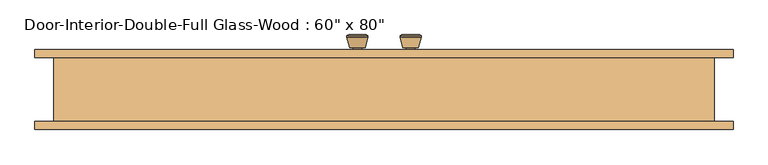
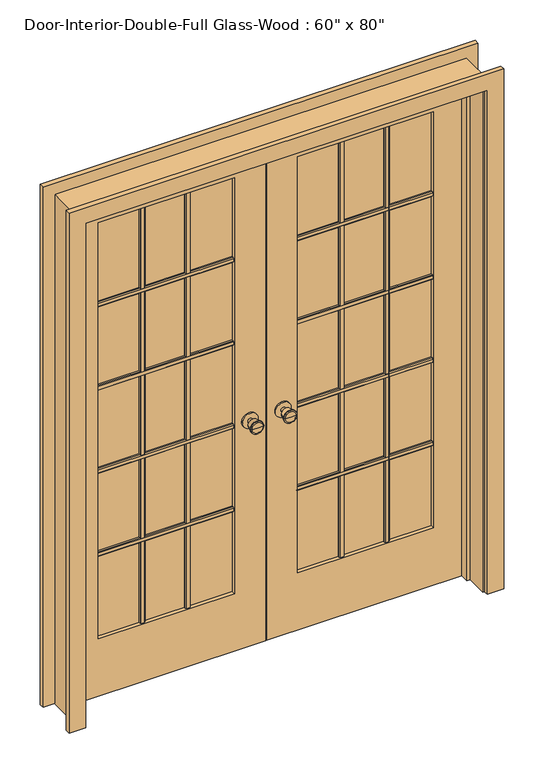
"""IFC4 building model written with IfcOpenShell, lengths in millimetres: door geometry."""

from ifc_helpers import new_model, si_unit, point, frame, frame_2d, origin, place, context, project, spatial, polyline, circle_curve, trimmed, segment, composite_curve, outline, extrude, faceted_brep, source, transform, mapped, element, save
from ifc_brep_helpers import plane_surface, cylinder_surface, revolved_surface, advanced_brep


def door_31a77bde(model_context):
    return source(origin(), model_context, "Body", "SolidModel", [
        advanced_brep(
        [(-63.5, 79.025, 914.4), (-73.5, 79.025, 914.4), (-53.5, 79.025, 914.4), (-83.9758676, 128.025, 914.4), (-63.5, 128.025, 914.4), (-43.0241324, 128.025, 914.4), (-88.5, 126.1971319, 914.4), (-38.5, 126.1971319, 914.4), (-88.5, 122.7334537, 914.4), (-38.5, 122.7334537, 914.4), (-82.136236, 98.025, 914.4), (-44.863764, 98.025, 914.4), (-73.5, 98.025, 914.4), (-53.5, 98.025, 914.4)],
        [
            (0, 1),
            (1, 2, circle_curve(frame((-63.5, 79.025, 914.4), z_axis=(0.0, -1.0, 0.0), x_axis=(1.0, 0.0, 0.0)), 10.0)),
            (2, 0),
            (2, 1, circle_curve(frame((-63.5, 79.025, 914.4), z_axis=(0.0, -1.0, 0.0), x_axis=(1.0, 0.0, 0.0)), 10.0)),
            (3, 4),
            (4, 5),
            (5, 3, circle_curve(frame((-63.5, 128.025, 914.4), z_axis=(0.0, 1.0, 0.0), x_axis=(1.0, 0.0, 0.0)), 20.4758676)),
            (3, 5, circle_curve(frame((-63.5, 128.025, 914.4), z_axis=(0.0, 1.0, 0.0), x_axis=(1.0, 0.0, 0.0)), 20.4758676)),
            (6, 3),
            (5, 7),
            (7, 6, circle_curve(frame((-63.5, 126.1971319, 914.4), z_axis=(0.0, 1.0, 0.0), x_axis=(1.0, 0.0, 0.0)), 25.0)),
            (6, 7, circle_curve(frame((-63.5, 126.1971319, 914.4), z_axis=(0.0, 1.0, 0.0), x_axis=(1.0, 0.0, 0.0)), 25.0)),
            (8, 6),
            (7, 9),
            (9, 8, circle_curve(frame((-63.5, 122.7334537, 914.4), z_axis=(0.0, 1.0, 0.0), x_axis=(1.0, 0.0, 0.0)), 25.0)),
            (8, 9, circle_curve(frame((-63.5, 122.7334537, 914.4), z_axis=(0.0, 1.0, 0.0), x_axis=(1.0, 0.0, 0.0)), 25.0)),
            (10, 8),
            (9, 11),
            (11, 10, circle_curve(frame((-63.5, 98.025, 914.4), z_axis=(0.0, 1.0, 0.0), x_axis=(1.0, 0.0, 0.0)), 18.636236)),
            (10, 11, circle_curve(frame((-63.5, 98.025, 914.4), z_axis=(0.0, 1.0, 0.0), x_axis=(1.0, 0.0, 0.0)), 18.636236)),
            (12, 10),
            (11, 13),
            (13, 12, circle_curve(frame((-63.5, 98.025, 914.4), z_axis=(0.0, 1.0, 0.0), x_axis=(1.0, 0.0, 0.0)), 10.0)),
            (12, 13, circle_curve(frame((-63.5, 98.025, 914.4), z_axis=(0.0, 1.0, 0.0), x_axis=(1.0, 0.0, 0.0)), 10.0)),
            (1, 12),
            (13, 2),
        ],
        [
            plane_surface(frame((-63.5, 79.025, 914.4), z_axis=(0.0, -1.0, 0.0), x_axis=(1.0, 0.0, 0.0))),
            plane_surface(frame((-63.5, 128.025, 914.4), z_axis=(0.0, 1.0, 0.0), x_axis=(1.0, 0.0, 0.0))),
            revolved_surface(polyline([(-43.0241324, 128.025, 914.4), (-38.5, 126.1971319, 914.4)]), (-63.5, 79.025, 914.4), (0.0, -1.0, 0.0)),
            cylinder_surface(frame((-63.5, 79.025, 914.4), z_axis=(0.0, -1.0, 0.0), x_axis=(1.0, 0.0, 0.0)), 25.0),
            revolved_surface(polyline([(-38.5, 122.7334537, 914.4), (-44.863764, 98.025, 914.4)]), (-63.5, 79.025, 914.4), (0.0, -1.0, 0.0)),
            plane_surface(frame((-63.5, 98.025, 914.4), z_axis=(0.0, -1.0, 0.0), x_axis=(1.0, 0.0, 0.0))),
            cylinder_surface(frame((-63.5, 79.025, 914.4), z_axis=(0.0, -1.0, 0.0), x_axis=(1.0, 0.0, 0.0)), 10.0),
        ],
        [
            (0, [[1, 2, 3]]),
            (0, [[-3, 4, -1]]),
            (1, [[5, 6, 7]]),
            (1, [[-6, -5, 8]]),
            (2, [[9, -7, 10, 11]]),
            (2, [[-10, -8, -9, 12]]),
            (3, [[13, -11, 14, 15]]),
            (3, [[-14, -12, -13, 16]]),
            (4, [[17, -15, 18, 19]]),
            (4, [[-18, -16, -17, 20]]),
            (5, [[21, -19, 22, 23]]),
            (5, [[-22, -20, -21, 24]]),
            (6, [[25, -23, 26, -2]]),
            (6, [[-26, -24, -25, -4]]),
        ],
    ),
        extrude(outline(composite_curve([segment(trimmed(circle_curve(frame_2d((914.4, -63.5)), 30.0), [point((914.4, -33.5))], [point((914.4, -93.5))], False, "CARTESIAN"), True, "CONTINUOUS"), segment(trimmed(circle_curve(frame_2d((914.4, -63.5)), 30.0), [point((914.4, -93.5))], [point((914.4, -33.5))], False, "CARTESIAN"), True, "CONTINUOUS")], self_intersect=False)), frame((0.0, 73.025, 0.0), z_axis=(0.0, 1.0, 0.0), x_axis=(0.0, 0.0, 1.0)), (0.0, 0.0, 1.0), 6.0),
        advanced_brep(
        [(-63.5, 32.1, 914.4), (-53.5, 32.1, 914.4), (-73.5, 32.1, 914.4), (-83.9758676, -16.9, 914.4), (-43.0241324, -16.9, 914.4), (-63.5, -16.9, 914.4), (-88.5, -15.0721319, 914.4), (-38.5, -15.0721319, 914.4), (-88.5, -11.6084537, 914.4), (-38.5, -11.6084537, 914.4), (-82.136236, 13.1, 914.4), (-44.863764, 13.1, 914.4), (-73.5, 13.1, 914.4), (-53.5, 13.1, 914.4)],
        [
            (0, 1),
            (1, 2, circle_curve(frame((-63.5, 32.1, 914.4), z_axis=(0.0, 1.0, 0.0), x_axis=(1.0, 0.0, 0.0)), 10.0)),
            (2, 0),
            (2, 1, circle_curve(frame((-63.5, 32.1, 914.4), z_axis=(0.0, 1.0, 0.0), x_axis=(1.0, 0.0, 0.0)), 10.0)),
            (3, 4, circle_curve(frame((-63.5, -16.9, 914.4), z_axis=(0.0, -1.0, 0.0), x_axis=(1.0, 0.0, 0.0)), 20.4758676)),
            (4, 5),
            (5, 3),
            (4, 3, circle_curve(frame((-63.5, -16.9, 914.4), z_axis=(0.0, -1.0, 0.0), x_axis=(1.0, 0.0, 0.0)), 20.4758676)),
            (6, 7, circle_curve(frame((-63.5, -15.0721319, 914.4), z_axis=(0.0, -1.0, 0.0), x_axis=(1.0, 0.0, 0.0)), 25.0)),
            (7, 4),
            (3, 6),
            (7, 6, circle_curve(frame((-63.5, -15.0721319, 914.4), z_axis=(0.0, -1.0, 0.0), x_axis=(1.0, 0.0, 0.0)), 25.0)),
            (8, 9, circle_curve(frame((-63.5, -11.6084537, 914.4), z_axis=(0.0, -1.0, 0.0), x_axis=(1.0, 0.0, 0.0)), 25.0)),
            (9, 7),
            (6, 8),
            (9, 8, circle_curve(frame((-63.5, -11.6084537, 914.4), z_axis=(0.0, -1.0, 0.0), x_axis=(1.0, 0.0, 0.0)), 25.0)),
            (10, 11, circle_curve(frame((-63.5, 13.1, 914.4), z_axis=(0.0, -1.0, 0.0), x_axis=(1.0, 0.0, 0.0)), 18.636236)),
            (11, 9),
            (8, 10),
            (11, 10, circle_curve(frame((-63.5, 13.1, 914.4), z_axis=(0.0, -1.0, 0.0), x_axis=(1.0, 0.0, 0.0)), 18.636236)),
            (12, 13, circle_curve(frame((-63.5, 13.1, 914.4), z_axis=(0.0, -1.0, 0.0), x_axis=(1.0, 0.0, 0.0)), 10.0)),
            (13, 11),
            (10, 12),
            (13, 12, circle_curve(frame((-63.5, 13.1, 914.4), z_axis=(0.0, -1.0, 0.0), x_axis=(1.0, 0.0, 0.0)), 10.0)),
            (1, 13),
            (12, 2),
        ],
        [
            plane_surface(frame((-63.5, 32.1, 914.4), z_axis=(0.0, 1.0, 0.0), x_axis=(1.0, 0.0, 0.0))),
            plane_surface(frame((-63.5, -16.9, 914.4), z_axis=(0.0, -1.0, 0.0), x_axis=(1.0, 0.0, 0.0))),
            revolved_surface(polyline([(-43.0241324, -16.9, 914.4), (-38.5, -15.0721319, 914.4)]), (-63.5, 32.1, 914.4), (0.0, 1.0, 0.0)),
            cylinder_surface(frame((-63.5, 32.1, 914.4), z_axis=(0.0, 1.0, 0.0), x_axis=(1.0, 0.0, 0.0)), 25.0),
            revolved_surface(polyline([(-38.5, -11.6084537, 914.4), (-44.863764, 13.1, 914.4)]), (-63.5, 32.1, 914.4), (0.0, 1.0, 0.0)),
            plane_surface(frame((-63.5, 13.1, 914.4), z_axis=(0.0, 1.0, 0.0), x_axis=(1.0, 0.0, 0.0))),
            cylinder_surface(frame((-63.5, 32.1, 914.4), z_axis=(0.0, 1.0, 0.0), x_axis=(1.0, 0.0, 0.0)), 10.0),
        ],
        [
            (0, [[1, 2, 3]]),
            (0, [[-3, 4, -1]]),
            (1, [[5, 6, 7]]),
            (1, [[8, -7, -6]]),
            (2, [[9, 10, -5, 11]]),
            (2, [[12, -11, -8, -10]]),
            (3, [[13, 14, -9, 15]]),
            (3, [[16, -15, -12, -14]]),
            (4, [[17, 18, -13, 19]]),
            (4, [[20, -19, -16, -18]]),
            (5, [[21, 22, -17, 23]]),
            (5, [[24, -23, -20, -22]]),
            (6, [[-2, 25, -21, 26]]),
            (6, [[-4, -26, -24, -25]]),
        ],
    ),
        extrude(outline(composite_curve([segment(trimmed(circle_curve(frame_2d((914.4, -63.5)), 30.0), [point((914.4, -33.5))], [point((914.4, -93.5))], False, "CARTESIAN"), True, "CONTINUOUS"), segment(trimmed(circle_curve(frame_2d((914.4, -63.5)), 30.0), [point((914.4, -93.5))], [point((914.4, -33.5))], False, "CARTESIAN"), True, "CONTINUOUS")], self_intersect=False)), frame((0.0, 32.1, 0.0), z_axis=(0.0, 1.0, 0.0), x_axis=(0.0, 0.0, 1.0)), (0.0, 0.0, 1.0), 6.0),
        extrude(outline(polyline([(52.07, 1586.23), (52.07, 1567.18), (45.72, 1567.18), (42.545, 1570.355), (42.545, 1583.055), (45.72, 1586.23), (52.07, 1586.23)])), frame((120.65, 0.0, 0.0), z_axis=(1.0, 0.0, 0.0), x_axis=(0.0, 1.0, 0.0)), (0.0, 0.0, 1.0), 520.7),
        extrude(outline(polyline([(52.07, 1249.9975), (52.07, 1230.9475), (45.72, 1230.9475), (42.545, 1234.1225), (42.545, 1246.8225), (45.72, 1249.9975), (52.07, 1249.9975)])), frame((120.65, 0.0, 0.0), z_axis=(1.0, 0.0, 0.0), x_axis=(0.0, 1.0, 0.0)), (0.0, 0.0, 1.0), 520.7),
        extrude(outline(polyline([(52.07, 913.765), (52.07, 894.715), (45.72, 894.715), (42.545, 897.89), (42.545, 910.59), (45.72, 913.765), (52.07, 913.765)])), frame((120.65, 0.0, 0.0), z_axis=(1.0, 0.0, 0.0), x_axis=(0.0, 1.0, 0.0)), (0.0, 0.0, 1.0), 520.7),
        extrude(outline(polyline([(52.07, 577.5325), (52.07, 558.4825), (45.72, 558.4825), (42.545, 561.6575), (42.545, 574.3575), (45.72, 577.5325), (52.07, 577.5325)])), frame((120.65, 0.0, 0.0), z_axis=(1.0, 0.0, 0.0), x_axis=(0.0, 1.0, 0.0)), (0.0, 0.0, 1.0), 520.7),
        extrude(outline(polyline([(458.2583333, 52.07), (477.3083333, 52.07), (477.3083333, 45.72), (474.1333333, 42.545), (461.4333333, 42.545), (458.2583333, 45.72), (458.2583333, 52.07)])), frame((0.0, 0.0, 231.775), z_axis=(0.0, 0.0, 1.0), x_axis=(1.0, 0.0, 0.0)), (0.0, 0.0, 1.0), 1681.1625),
        extrude(outline(polyline([(284.6916667, 52.07), (303.7416667, 52.07), (303.7416667, 45.72), (300.5666667, 42.545), (287.8666667, 42.545), (284.6916667, 45.72), (284.6916667, 52.07)])), frame((0.0, 0.0, 231.775), z_axis=(0.0, 0.0, 1.0), x_axis=(1.0, 0.0, 0.0)), (0.0, 0.0, 1.0), 1681.1625),
        extrude(outline(polyline([(59.055, 1586.23), (65.405, 1586.23), (68.58, 1583.055), (68.58, 1570.355), (65.405, 1567.18), (59.055, 1567.18), (59.055, 1586.23)])), frame((-641.35, 0.0, 0.0), z_axis=(1.0, 0.0, 0.0), x_axis=(0.0, 1.0, 0.0)), (0.0, 0.0, 1.0), 520.7),
        extrude(outline(polyline([(59.055, 1249.9975), (65.405, 1249.9975), (68.58, 1246.8225), (68.58, 1234.1225), (65.405, 1230.9475), (59.055, 1230.9475), (59.055, 1249.9975)])), frame((-641.35, 0.0, 0.0), z_axis=(1.0, 0.0, 0.0), x_axis=(0.0, 1.0, 0.0)), (0.0, 0.0, 1.0), 520.7),
        extrude(outline(polyline([(59.055, 913.765), (65.405, 913.765), (68.58, 910.59), (68.58, 897.89), (65.405, 894.715), (59.055, 894.715), (59.055, 913.765)])), frame((-641.35, 0.0, 0.0), z_axis=(1.0, 0.0, 0.0), x_axis=(0.0, 1.0, 0.0)), (0.0, 0.0, 1.0), 520.7),
        extrude(outline(polyline([(59.055, 577.5325), (65.405, 577.5325), (68.58, 574.3575), (68.58, 561.6575), (65.405, 558.4825), (59.055, 558.4825), (59.055, 577.5325)])), frame((-641.35, 0.0, 0.0), z_axis=(1.0, 0.0, 0.0), x_axis=(0.0, 1.0, 0.0)), (0.0, 0.0, 1.0), 520.7),
        extrude(outline(polyline([(-303.7416667, 59.055), (-303.7416667, 65.405), (-300.5666667, 68.58), (-287.8666667, 68.58), (-284.6916667, 65.405), (-284.6916667, 59.055), (-303.7416667, 59.055)])), frame((0.0, 0.0, 231.775), z_axis=(0.0, 0.0, 1.0), x_axis=(1.0, 0.0, 0.0)), (0.0, 0.0, 1.0), 1681.1625),
        extrude(outline(polyline([(-477.3083333, 59.055), (-477.3083333, 65.405), (-474.1333333, 68.58), (-461.4333333, 68.58), (-458.2583333, 65.405), (-458.2583333, 59.055), (-477.3083333, 59.055)])), frame((0.0, 0.0, 231.775), z_axis=(0.0, 0.0, 1.0), x_axis=(1.0, 0.0, 0.0)), (0.0, 0.0, 1.0), 1681.1625),
        extrude(outline(polyline([(59.055, 1586.23), (65.405, 1586.23), (68.58, 1583.055), (68.58, 1570.355), (65.405, 1567.18), (59.055, 1567.18), (59.055, 1586.23)])), frame((120.65, 0.0, 0.0), z_axis=(1.0, 0.0, 0.0), x_axis=(0.0, 1.0, 0.0)), (0.0, 0.0, 1.0), 520.7),
        extrude(outline(polyline([(59.055, 1249.9975), (65.405, 1249.9975), (68.58, 1246.8225), (68.58, 1234.1225), (65.405, 1230.9475), (59.055, 1230.9475), (59.055, 1249.9975)])), frame((120.65, 0.0, 0.0), z_axis=(1.0, 0.0, 0.0), x_axis=(0.0, 1.0, 0.0)), (0.0, 0.0, 1.0), 520.7),
        extrude(outline(polyline([(59.055, 913.765), (65.405, 913.765), (68.58, 910.59), (68.58, 897.89), (65.405, 894.715), (59.055, 894.715), (59.055, 913.765)])), frame((120.65, 0.0, 0.0), z_axis=(1.0, 0.0, 0.0), x_axis=(0.0, 1.0, 0.0)), (0.0, 0.0, 1.0), 520.7),
        extrude(outline(polyline([(59.055, 577.5325), (65.405, 577.5325), (68.58, 574.3575), (68.58, 561.6575), (65.405, 558.4825), (59.055, 558.4825), (59.055, 577.5325)])), frame((120.65, 0.0, 0.0), z_axis=(1.0, 0.0, 0.0), x_axis=(0.0, 1.0, 0.0)), (0.0, 0.0, 1.0), 520.7),
        extrude(outline(polyline([(458.2583333, 59.055), (458.2583333, 65.405), (461.4333333, 68.58), (474.1333333, 68.58), (477.3083333, 65.405), (477.3083333, 59.055), (458.2583333, 59.055)])), frame((0.0, 0.0, 231.775), z_axis=(0.0, 0.0, 1.0), x_axis=(1.0, 0.0, 0.0)), (0.0, 0.0, 1.0), 1681.1625),
        extrude(outline(polyline([(284.6916667, 59.055), (284.6916667, 65.405), (287.8666667, 68.58), (300.5666667, 68.58), (303.7416667, 65.405), (303.7416667, 59.055), (284.6916667, 59.055)])), frame((0.0, 0.0, 231.775), z_axis=(0.0, 0.0, 1.0), x_axis=(1.0, 0.0, 0.0)), (0.0, 0.0, 1.0), 1681.1625),
        extrude(outline(polyline([(52.07, 1586.23), (52.07, 1567.18), (45.72, 1567.18), (42.545, 1570.355), (42.545, 1583.055), (45.72, 1586.23), (52.07, 1586.23)])), frame((-641.35, 0.0, 0.0), z_axis=(1.0, 0.0, 0.0), x_axis=(0.0, 1.0, 0.0)), (0.0, 0.0, 1.0), 520.7),
        extrude(outline(polyline([(52.07, 1249.9975), (52.07, 1230.9475), (45.72, 1230.9475), (42.545, 1234.1225), (42.545, 1246.8225), (45.72, 1249.9975), (52.07, 1249.9975)])), frame((-641.35, 0.0, 0.0), z_axis=(1.0, 0.0, 0.0), x_axis=(0.0, 1.0, 0.0)), (0.0, 0.0, 1.0), 520.7),
        extrude(outline(polyline([(52.07, 913.765), (52.07, 894.715), (45.72, 894.715), (42.545, 897.89), (42.545, 910.59), (45.72, 913.765), (52.07, 913.765)])), frame((-641.35, 0.0, 0.0), z_axis=(1.0, 0.0, 0.0), x_axis=(0.0, 1.0, 0.0)), (0.0, 0.0, 1.0), 520.7),
        extrude(outline(polyline([(52.07, 577.5325), (52.07, 558.4825), (45.72, 558.4825), (42.545, 561.6575), (42.545, 574.3575), (45.72, 577.5325), (52.07, 577.5325)])), frame((-641.35, 0.0, 0.0), z_axis=(1.0, 0.0, 0.0), x_axis=(0.0, 1.0, 0.0)), (0.0, 0.0, 1.0), 520.7),
        extrude(outline(polyline([(-303.7416667, 52.07), (-284.6916667, 52.07), (-284.6916667, 45.72), (-287.8666667, 42.545), (-300.5666667, 42.545), (-303.7416667, 45.72), (-303.7416667, 52.07)])), frame((0.0, 0.0, 231.775), z_axis=(0.0, 0.0, 1.0), x_axis=(1.0, 0.0, 0.0)), (0.0, 0.0, 1.0), 1681.1625),
        extrude(outline(polyline([(-477.3083333, 52.07), (-458.2583333, 52.07), (-458.2583333, 45.72), (-461.4333333, 42.545), (-474.1333333, 42.545), (-477.3083333, 45.72), (-477.3083333, 52.07)])), frame((0.0, 0.0, 231.775), z_axis=(0.0, 0.0, 1.0), x_axis=(1.0, 0.0, 0.0)), (0.0, 0.0, 1.0), 1681.1625),
        advanced_brep(
        [(63.5, 32.1, 914.4), (73.5, 32.1, 914.4), (53.5, 32.1, 914.4), (83.9758676, -16.9, 914.4), (63.5, -16.9, 914.4), (43.0241324, -16.9, 914.4), (88.5, -15.0721319, 914.4), (38.5, -15.0721319, 914.4), (88.5, -11.6084537, 914.4), (38.5, -11.6084537, 914.4), (82.136236, 13.1, 914.4), (44.863764, 13.1, 914.4), (73.5, 13.1, 914.4), (53.5, 13.1, 914.4)],
        [
            (0, 1),
            (1, 2, circle_curve(frame((63.5, 32.1, 914.4), z_axis=(0.0, 1.0, 0.0), x_axis=(-1.0, 0.0, 0.0)), 10.0)),
            (2, 0),
            (2, 1, circle_curve(frame((63.5, 32.1, 914.4), z_axis=(0.0, 1.0, 0.0), x_axis=(-1.0, 0.0, 0.0)), 10.0)),
            (3, 4),
            (4, 5),
            (5, 3, circle_curve(frame((63.5, -16.9, 914.4), z_axis=(0.0, -1.0, 0.0), x_axis=(-1.0, 0.0, 0.0)), 20.4758676)),
            (3, 5, circle_curve(frame((63.5, -16.9, 914.4), z_axis=(0.0, -1.0, 0.0), x_axis=(-1.0, 0.0, 0.0)), 20.4758676)),
            (6, 3),
            (5, 7),
            (7, 6, circle_curve(frame((63.5, -15.0721319, 914.4), z_axis=(0.0, -1.0, 0.0), x_axis=(-1.0, 0.0, 0.0)), 25.0)),
            (6, 7, circle_curve(frame((63.5, -15.0721319, 914.4), z_axis=(0.0, -1.0, 0.0), x_axis=(-1.0, 0.0, 0.0)), 25.0)),
            (8, 6),
            (7, 9),
            (9, 8, circle_curve(frame((63.5, -11.6084537, 914.4), z_axis=(0.0, -1.0, 0.0), x_axis=(-1.0, 0.0, 0.0)), 25.0)),
            (8, 9, circle_curve(frame((63.5, -11.6084537, 914.4), z_axis=(0.0, -1.0, 0.0), x_axis=(-1.0, 0.0, 0.0)), 25.0)),
            (10, 8),
            (9, 11),
            (11, 10, circle_curve(frame((63.5, 13.1, 914.4), z_axis=(0.0, -1.0, 0.0), x_axis=(-1.0, 0.0, 0.0)), 18.636236)),
            (10, 11, circle_curve(frame((63.5, 13.1, 914.4), z_axis=(0.0, -1.0, 0.0), x_axis=(-1.0, 0.0, 0.0)), 18.636236)),
            (12, 10),
            (11, 13),
            (13, 12, circle_curve(frame((63.5, 13.1, 914.4), z_axis=(0.0, -1.0, 0.0), x_axis=(-1.0, 0.0, 0.0)), 10.0)),
            (12, 13, circle_curve(frame((63.5, 13.1, 914.4), z_axis=(0.0, -1.0, 0.0), x_axis=(-1.0, 0.0, 0.0)), 10.0)),
            (1, 12),
            (13, 2),
        ],
        [
            plane_surface(frame((63.5, 32.1, 914.4), z_axis=(0.0, 1.0, 0.0), x_axis=(-1.0, 0.0, 0.0))),
            plane_surface(frame((63.5, -16.9, 914.4), z_axis=(0.0, -1.0, 0.0), x_axis=(-1.0, 0.0, 0.0))),
            revolved_surface(polyline([(43.0241324, -16.9, 914.4), (38.5, -15.0721319, 914.4)]), (63.5, 32.1, 914.4), (0.0, 1.0, 0.0)),
            cylinder_surface(frame((63.5, 32.1, 914.4), z_axis=(0.0, 1.0, 0.0), x_axis=(-1.0, 0.0, 0.0)), 25.0),
            revolved_surface(polyline([(38.5, -11.6084537, 914.4), (44.863764, 13.1, 914.4)]), (63.5, 32.1, 914.4), (0.0, 1.0, 0.0)),
            plane_surface(frame((63.5, 13.1, 914.4), z_axis=(0.0, 1.0, 0.0), x_axis=(-1.0, 0.0, 0.0))),
            cylinder_surface(frame((63.5, 32.1, 914.4), z_axis=(0.0, 1.0, 0.0), x_axis=(-1.0, 0.0, 0.0)), 10.0),
        ],
        [
            (0, [[1, 2, 3]]),
            (0, [[-3, 4, -1]]),
            (1, [[5, 6, 7]]),
            (1, [[-6, -5, 8]]),
            (2, [[9, -7, 10, 11]]),
            (2, [[-10, -8, -9, 12]]),
            (3, [[13, -11, 14, 15]]),
            (3, [[-14, -12, -13, 16]]),
            (4, [[17, -15, 18, 19]]),
            (4, [[-18, -16, -17, 20]]),
            (5, [[21, -19, 22, 23]]),
            (5, [[-22, -20, -21, 24]]),
            (6, [[25, -23, 26, -2]]),
            (6, [[-26, -24, -25, -4]]),
        ],
    ),
        extrude(outline(composite_curve([segment(trimmed(circle_curve(frame_2d((914.4, 63.5)), 30.0), [point((914.4, 33.5))], [point((914.4, 93.5))], False, "CARTESIAN"), True, "CONTINUOUS"), segment(trimmed(circle_curve(frame_2d((914.4, 63.5)), 30.0), [point((914.4, 93.5))], [point((914.4, 33.5))], False, "CARTESIAN"), True, "CONTINUOUS")], self_intersect=False)), frame((0.0, 32.1, 0.0), z_axis=(0.0, 1.0, 0.0), x_axis=(0.0, 0.0, 1.0)), (0.0, 0.0, 1.0), 6.0),
        advanced_brep(
        [(63.5, 79.025, 914.4), (53.5, 79.025, 914.4), (73.5, 79.025, 914.4), (83.9758676, 128.025, 914.4), (43.0241324, 128.025, 914.4), (63.5, 128.025, 914.4), (88.5, 126.1971319, 914.4), (38.5, 126.1971319, 914.4), (88.5, 122.7334537, 914.4), (38.5, 122.7334537, 914.4), (82.136236, 98.025, 914.4), (44.863764, 98.025, 914.4), (73.5, 98.025, 914.4), (53.5, 98.025, 914.4)],
        [
            (0, 1),
            (1, 2, circle_curve(frame((63.5, 79.025, 914.4), z_axis=(0.0, -1.0, 0.0), x_axis=(-1.0, 0.0, 0.0)), 10.0)),
            (2, 0),
            (2, 1, circle_curve(frame((63.5, 79.025, 914.4), z_axis=(0.0, -1.0, 0.0), x_axis=(-1.0, 0.0, 0.0)), 10.0)),
            (3, 4, circle_curve(frame((63.5, 128.025, 914.4), z_axis=(0.0, 1.0, 0.0), x_axis=(-1.0, 0.0, 0.0)), 20.4758676)),
            (4, 5),
            (5, 3),
            (4, 3, circle_curve(frame((63.5, 128.025, 914.4), z_axis=(0.0, 1.0, 0.0), x_axis=(-1.0, 0.0, 0.0)), 20.4758676)),
            (6, 7, circle_curve(frame((63.5, 126.1971319, 914.4), z_axis=(0.0, 1.0, 0.0), x_axis=(-1.0, 0.0, 0.0)), 25.0)),
            (7, 4),
            (3, 6),
            (7, 6, circle_curve(frame((63.5, 126.1971319, 914.4), z_axis=(0.0, 1.0, 0.0), x_axis=(-1.0, 0.0, 0.0)), 25.0)),
            (8, 9, circle_curve(frame((63.5, 122.7334537, 914.4), z_axis=(0.0, 1.0, 0.0), x_axis=(-1.0, 0.0, 0.0)), 25.0)),
            (9, 7),
            (6, 8),
            (9, 8, circle_curve(frame((63.5, 122.7334537, 914.4), z_axis=(0.0, 1.0, 0.0), x_axis=(-1.0, 0.0, 0.0)), 25.0)),
            (10, 11, circle_curve(frame((63.5, 98.025, 914.4), z_axis=(0.0, 1.0, 0.0), x_axis=(-1.0, 0.0, 0.0)), 18.636236)),
            (11, 9),
            (8, 10),
            (11, 10, circle_curve(frame((63.5, 98.025, 914.4), z_axis=(0.0, 1.0, 0.0), x_axis=(-1.0, 0.0, 0.0)), 18.636236)),
            (12, 13, circle_curve(frame((63.5, 98.025, 914.4), z_axis=(0.0, 1.0, 0.0), x_axis=(-1.0, 0.0, 0.0)), 10.0)),
            (13, 11),
            (10, 12),
            (13, 12, circle_curve(frame((63.5, 98.025, 914.4), z_axis=(0.0, 1.0, 0.0), x_axis=(-1.0, 0.0, 0.0)), 10.0)),
            (1, 13),
            (12, 2),
        ],
        [
            plane_surface(frame((63.5, 79.025, 914.4), z_axis=(0.0, -1.0, 0.0), x_axis=(-1.0, 0.0, 0.0))),
            plane_surface(frame((63.5, 128.025, 914.4), z_axis=(0.0, 1.0, 0.0), x_axis=(-1.0, 0.0, 0.0))),
            revolved_surface(polyline([(43.0241324, 128.025, 914.4), (38.5, 126.1971319, 914.4)]), (63.5, 79.025, 914.4), (0.0, -1.0, 0.0)),
            cylinder_surface(frame((63.5, 79.025, 914.4), z_axis=(0.0, -1.0, 0.0), x_axis=(-1.0, 0.0, 0.0)), 25.0),
            revolved_surface(polyline([(38.5, 122.7334537, 914.4), (44.863764, 98.025, 914.4)]), (63.5, 79.025, 914.4), (0.0, -1.0, 0.0)),
            plane_surface(frame((63.5, 98.025, 914.4), z_axis=(0.0, -1.0, 0.0), x_axis=(-1.0, 0.0, 0.0))),
            cylinder_surface(frame((63.5, 79.025, 914.4), z_axis=(0.0, -1.0, 0.0), x_axis=(-1.0, 0.0, 0.0)), 10.0),
        ],
        [
            (0, [[1, 2, 3]]),
            (0, [[-3, 4, -1]]),
            (1, [[5, 6, 7]]),
            (1, [[8, -7, -6]]),
            (2, [[9, 10, -5, 11]]),
            (2, [[12, -11, -8, -10]]),
            (3, [[13, 14, -9, 15]]),
            (3, [[16, -15, -12, -14]]),
            (4, [[17, 18, -13, 19]]),
            (4, [[20, -19, -16, -18]]),
            (5, [[21, 22, -17, 23]]),
            (5, [[24, -23, -20, -22]]),
            (6, [[-2, 25, -21, 26]]),
            (6, [[-4, -26, -24, -25]]),
        ],
    ),
        extrude(outline(composite_curve([segment(trimmed(circle_curve(frame_2d((914.4, 63.5)), 30.0), [point((914.4, 33.5))], [point((914.4, 93.5))], False, "CARTESIAN"), True, "CONTINUOUS"), segment(trimmed(circle_curve(frame_2d((914.4, 63.5)), 30.0), [point((914.4, 93.5))], [point((914.4, 33.5))], False, "CARTESIAN"), True, "CONTINUOUS")], self_intersect=False)), frame((0.0, 73.025, 0.0), z_axis=(0.0, 1.0, 0.0), x_axis=(0.0, 0.0, 1.0)), (0.0, 0.0, 1.0), 6.0),
        extrude(outline(polyline([(0.0, 768.35), (0.0, 831.85), (2101.85, 831.85), (2101.85, -831.85), (0.0, -831.85), (0.0, -768.35), (2038.35, -768.35), (2038.35, 768.35), (0.0, 768.35)])), frame((0.0, 73.025, 0.0), z_axis=(0.0, 1.0, 0.0), x_axis=(0.0, 0.0, 1.0)), (0.0, 0.0, 1.0), 19.05),
        extrude(outline(polyline([(0.0, 768.35), (0.0, 831.85), (2101.85, 831.85), (2101.85, -831.85), (0.0, -831.85), (0.0, -768.35), (2038.35, -768.35), (2038.35, 768.35), (0.0, 768.35)])), frame((0.0, -98.425, 0.0), z_axis=(0.0, 1.0, 0.0), x_axis=(0.0, 0.0, 1.0)), (0.0, 0.0, 1.0), 19.05),
        extrude(outline(polyline([(2032.0, -762.0), (0.0, -762.0), (0.0, -1.6019111), (2032.0, -1.6019111), (2032.0, -762.0)]), holes=[polyline([(231.775, -641.35), (1912.9375, -641.35), (1912.9375, -120.65), (231.775, -120.65), (231.775, -641.35)])]), frame((0.0, 38.1, 0.0), z_axis=(0.0, 1.0, 0.0), x_axis=(0.0, 0.0, 1.0)), (0.0, 0.0, 1.0), 34.925),
        extrude(outline(polyline([(0.0, 762.0), (2032.0, 762.0), (2032.0, 1.5875), (0.0, 1.5875), (0.0, 762.0)]), holes=[polyline([(1912.9375, 120.65), (1912.9375, 641.35), (231.775, 641.35), (231.775, 120.65), (1912.9375, 120.65)])]), frame((0.0, 38.1, 0.0), z_axis=(0.0, 1.0, 0.0), x_axis=(0.0, 0.0, 1.0)), (0.0, 0.0, 1.0), 34.925),
        faceted_brep([(787.4, 73.025, 0.0), (787.4, -79.375, 0.0), (762.0, -79.375, 0.0), (762.0, 3.175, 0.0), (749.3, 3.175, 0.0), (749.3, 38.1, 0.0), (762.0, 38.1, 0.0), (762.0, 73.025, 0.0), (787.4, 73.025, 2057.4), (787.4, -79.375, 2057.4), (-787.4, -79.375, 2057.4), (-787.4, -79.375, 0.0), (-762.0, -79.375, 0.0), (-762.0, -79.375, 2032.0), (762.0, -79.375, 2032.0), (762.0, 3.175, 2032.0), (-762.0, 3.175, 2032.0), (-762.0, 3.175, 0.0), (-749.3, 3.175, 0.0), (-749.3, 3.175, 2019.3), (749.3, 3.175, 2019.3), (749.3, 38.1, 2019.3), (1.5875, 38.1, 2019.3), (-1.6019111, 38.1, 2019.3), (-749.3, 38.1, 2019.3), (-749.3, 38.1, 0.0), (-762.0, 38.1, 0.0), (-762.0, 38.1, 2032.0), (-1.6019111, 38.1, 2032.0), (1.5875, 38.1, 2032.0), (762.0, 38.1, 2032.0), (762.0, 73.025, 2032.0), (1.5875, 73.025, 2032.0), (-1.6019111, 73.025, 2032.0), (-762.0, 73.025, 2032.0), (-762.0, 73.025, 0.0), (-787.4, 73.025, 0.0), (-787.4, 73.025, 2057.4)], [[[0, 1, 2, 3, 4, 5, 6, 7]], [[1, 0, 8, 9]], [[2, 1, 9, 10, 11, 12, 13, 14]], [[3, 2, 14, 15]], [[4, 3, 15, 16, 17, 18, 19, 20]], [[5, 4, 20, 21]], [[6, 5, 21, 22, 23, 24, 25, 26, 27, 28, 29, 30]], [[7, 6, 30, 31]], [[0, 7, 31, 32, 33, 34, 35, 36, 37, 8]], [[9, 8, 37, 10]], [[14, 13, 16, 15]], [[20, 19, 24, 23, 22, 21]], [[31, 30, 29, 28, 27, 34, 33, 32]], [[12, 11, 36, 35, 26, 25, 18, 17]], [[11, 10, 37, 36]], [[13, 12, 17, 16]], [[19, 18, 25, 24]], [[27, 26, 35, 34]]]),
        extrude(outline(polyline([(641.35, 52.07), (120.65, 52.07), (120.65, 59.055), (641.35, 59.055), (641.35, 52.07)])), frame((0.0, 0.0, 231.775), z_axis=(0.0, 0.0, 1.0), x_axis=(1.0, 0.0, 0.0)), (0.0, 0.0, 1.0), 1681.1625),
        extrude(outline(polyline([(-120.65, 52.07), (-641.35, 52.07), (-641.35, 59.055), (-120.65, 59.055), (-120.65, 52.07)])), frame((0.0, 0.0, 231.775), z_axis=(0.0, 0.0, 1.0), x_axis=(1.0, 0.0, 0.0)), (0.0, 0.0, 1.0), 1681.1625),
    ])


if __name__ == "__main__":
    model = new_model("IFC4")
    model_context = context("Model", 3, world=origin())
    ifc_project = project(units=[si_unit("LENGTHUNIT", "METRE", prefix="MILLI")], contexts=[model_context])
    site = spatial("IfcSite", under=ifc_project)
    building = spatial("IfcBuilding", under=site)
    placement = place(None, origin())
    door_shape = door_31a77bde(model_context)
    element("IfcDoor", 1, ObjectType="Door-Interior-Double-Full Glass-Wood : 60\" x 80\"", at=placement, inside=building, context=model_context, shape_type="MappedRepresentation", body=[
        mapped(door_shape, transform((0.0, 0.0, 0.0), x_axis=(1.0, 0.0, 0.0), y_axis=(0.0, 1.0, 0.0), z_axis=(0.0, 0.0, 1.0))),
    ])
    save(model, "model.ifc")

# Revit data of these elements
# Type "Door-Interior-Double-Full Glass-Wood : 60\" x 80\""
#   Type Mark = "8"
#   Assembly Code = "C1020300"
#   Analytic Construction = "French door, wood frame with single glass"
#   Top Rail = 0' - 4 11/16"
#   Thickness = 0' - 1 3/8"
#   Thermal Resistance (R) = 1.0696 (h·ft²·°F)/BTU
#   Swing Angle [instance default] = 90.00°
#   Stiles = 0' - 4 3/4"
#   Rough Width = 5' - 2"
#   Rough Height = 6' - 9"
#   Panel Width = 2' - 6"
#   Height = 6' - 8"
#   Width = 5' - 0"
#   Heat Transfer Coefficient (U) = 0.9350 BTU/(h·ft²·°F)
#   Bottom Rail = 0' - 9 1/8"
#   Show Grill [instance default] = yes
#   Trim Material = Cherry
#   Panel Material = Cherry
#   Frame Material = Cherry
#   Door Handle Material = Aluminum
#   Visual Light Transmittance = 0
#   Solar Heat Gain Coefficient = 0
#   Wall Closure = (empty or 0)
#   Function = (empty or 0)
# Element 1 (IfcDoor, "Door-Interior-Double-Full Glass-Wood : 60\" x 80\"")
#   Materials on its faces: "Cherry", "Aluminum", "Glass"
# Materials
#   "Cherry": class "Wood", colour RGB 226 177 128, transparency 0, Description = "Prunus Serotina", Cost = 0
#   "Aluminum": class "Metal", colour RGB 247 247 247, transparency 0, Description = "Aluminum 6061", Cost = 0
#   "Glass": class "Glass", colour RGB 0 128 192, transparency 0.75, Description = "Soda Lime Glass", Cost = 0
